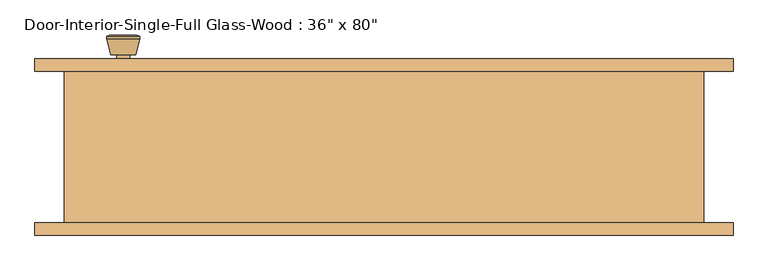
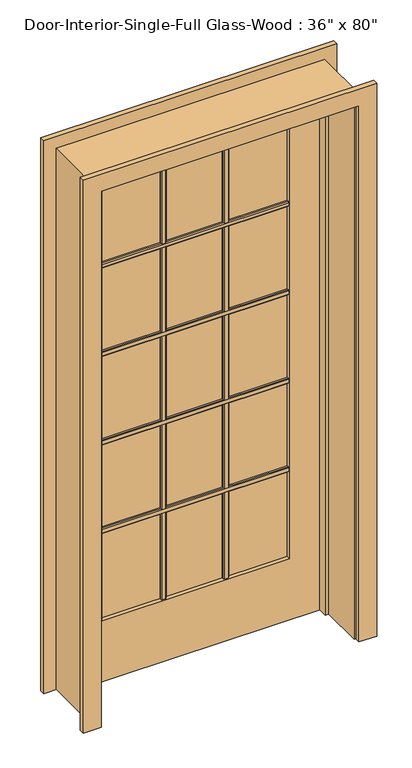
"""IFC4 building model written with IfcOpenShell, lengths in millimetres: door geometry."""

from ifc_helpers import new_model, si_unit, point, frame, frame_2d, origin, place, context, project, spatial, polyline, circle_curve, trimmed, segment, composite_curve, outline, extrude, faceted_brep, source, transform, mapped, element, save
from ifc_brep_helpers import plane_surface, cylinder_surface, revolved_surface, advanced_brep


def door_d5d480c1(model_context):
    return source(origin(), model_context, "Body", "SolidModel", [
        extrude(outline(polyline([(97.155, 1586.23), (103.505, 1586.23), (106.68, 1583.055), (106.68, 1570.355), (103.505, 1567.18), (97.155, 1567.18), (97.155, 1586.23)])), frame((-336.55, 0.0, 0.0), z_axis=(1.0, 0.0, 0.0), x_axis=(0.0, 1.0, 0.0)), (0.0, 0.0, 1.0), 673.1),
        extrude(outline(polyline([(97.155, 1249.9975), (103.505, 1249.9975), (106.68, 1246.8225), (106.68, 1234.1225), (103.505, 1230.9475), (97.155, 1230.9475), (97.155, 1249.9975)])), frame((-336.55, 0.0, 0.0), z_axis=(1.0, 0.0, 0.0), x_axis=(0.0, 1.0, 0.0)), (0.0, 0.0, 1.0), 673.1),
        extrude(outline(polyline([(97.155, 913.765), (103.505, 913.765), (106.68, 910.59), (106.68, 897.89), (103.505, 894.715), (97.155, 894.715), (97.155, 913.765)])), frame((-336.55, 0.0, 0.0), z_axis=(1.0, 0.0, 0.0), x_axis=(0.0, 1.0, 0.0)), (0.0, 0.0, 1.0), 673.1),
        extrude(outline(polyline([(97.155, 577.5325), (103.505, 577.5325), (106.68, 574.3575), (106.68, 561.6575), (103.505, 558.4825), (97.155, 558.4825), (97.155, 577.5325)])), frame((-336.55, 0.0, 0.0), z_axis=(1.0, 0.0, 0.0), x_axis=(0.0, 1.0, 0.0)), (0.0, 0.0, 1.0), 673.1),
        extrude(outline(polyline([(102.6583333, 97.155), (102.6583333, 103.505), (105.8333333, 106.68), (118.5333333, 106.68), (121.7083333, 103.505), (121.7083333, 97.155), (102.6583333, 97.155)])), frame((0.0, 0.0, 231.775), z_axis=(0.0, 0.0, 1.0), x_axis=(1.0, 0.0, 0.0)), (0.0, 0.0, 1.0), 1681.1625),
        extrude(outline(polyline([(-121.7083333, 97.155), (-121.7083333, 103.505), (-118.5333333, 106.68), (-105.8333333, 106.68), (-102.6583333, 103.505), (-102.6583333, 97.155), (-121.7083333, 97.155)])), frame((0.0, 0.0, 231.775), z_axis=(0.0, 0.0, 1.0), x_axis=(1.0, 0.0, 0.0)), (0.0, 0.0, 1.0), 1681.1625),
        extrude(outline(polyline([(90.17, 1586.23), (90.17, 1567.18), (83.82, 1567.18), (80.645, 1570.355), (80.645, 1583.055), (83.82, 1586.23), (90.17, 1586.23)])), frame((-336.55, 0.0, 0.0), z_axis=(1.0, 0.0, 0.0), x_axis=(0.0, 1.0, 0.0)), (0.0, 0.0, 1.0), 673.1),
        extrude(outline(polyline([(90.17, 1249.9975), (90.17, 1230.9475), (83.82, 1230.9475), (80.645, 1234.1225), (80.645, 1246.8225), (83.82, 1249.9975), (90.17, 1249.9975)])), frame((-336.55, 0.0, 0.0), z_axis=(1.0, 0.0, 0.0), x_axis=(0.0, 1.0, 0.0)), (0.0, 0.0, 1.0), 673.1),
        extrude(outline(polyline([(90.17, 913.765), (90.17, 894.715), (83.82, 894.715), (80.645, 897.89), (80.645, 910.59), (83.82, 913.765), (90.17, 913.765)])), frame((-336.55, 0.0, 0.0), z_axis=(1.0, 0.0, 0.0), x_axis=(0.0, 1.0, 0.0)), (0.0, 0.0, 1.0), 673.1),
        extrude(outline(polyline([(90.17, 577.5325), (90.17, 558.4825), (83.82, 558.4825), (80.645, 561.6575), (80.645, 574.3575), (83.82, 577.5325), (90.17, 577.5325)])), frame((-336.55, 0.0, 0.0), z_axis=(1.0, 0.0, 0.0), x_axis=(0.0, 1.0, 0.0)), (0.0, 0.0, 1.0), 673.1),
        extrude(outline(polyline([(102.6583333, 90.17), (121.7083333, 90.17), (121.7083333, 83.82), (118.5333333, 80.645), (105.8333333, 80.645), (102.6583333, 83.82), (102.6583333, 90.17)])), frame((0.0, 0.0, 231.775), z_axis=(0.0, 0.0, 1.0), x_axis=(1.0, 0.0, 0.0)), (0.0, 0.0, 1.0), 1681.1625),
        extrude(outline(polyline([(-121.7083333, 90.17), (-102.6583333, 90.17), (-102.6583333, 83.82), (-105.8333333, 80.645), (-118.5333333, 80.645), (-121.7083333, 83.82), (-121.7083333, 90.17)])), frame((0.0, 0.0, 231.775), z_axis=(0.0, 0.0, 1.0), x_axis=(1.0, 0.0, 0.0)), (0.0, 0.0, 1.0), 1681.1625),
        advanced_brep(
        [(-393.7, 70.2, 914.4), (-383.7, 70.2, 914.4), (-403.7, 70.2, 914.4), (-373.2241324, 21.2, 914.4), (-393.7, 21.2, 914.4), (-414.1758676, 21.2, 914.4), (-368.7, 23.0278681, 914.4), (-418.7, 23.0278681, 914.4), (-368.7, 26.4915463, 914.4), (-418.7, 26.4915463, 914.4), (-375.063764, 51.2, 914.4), (-412.336236, 51.2, 914.4), (-383.7, 51.2, 914.4), (-403.7, 51.2, 914.4)],
        [
            (0, 1),
            (1, 2, circle_curve(frame((-393.7, 70.2, 914.4), z_axis=(0.0, 1.0, 0.0), x_axis=(-1.0, 0.0, 0.0)), 10.0)),
            (2, 0),
            (2, 1, circle_curve(frame((-393.7, 70.2, 914.4), z_axis=(0.0, 1.0, 0.0), x_axis=(-1.0, 0.0, 0.0)), 10.0)),
            (3, 4),
            (4, 5),
            (5, 3, circle_curve(frame((-393.7, 21.2, 914.4), z_axis=(0.0, -1.0, 0.0), x_axis=(-1.0, 0.0, 0.0)), 20.4758676)),
            (3, 5, circle_curve(frame((-393.7, 21.2, 914.4), z_axis=(0.0, -1.0, 0.0), x_axis=(-1.0, 0.0, 0.0)), 20.4758676)),
            (6, 3),
            (5, 7),
            (7, 6, circle_curve(frame((-393.7, 23.0278681, 914.4), z_axis=(0.0, -1.0, 0.0), x_axis=(-1.0, 0.0, 0.0)), 25.0)),
            (6, 7, circle_curve(frame((-393.7, 23.0278681, 914.4), z_axis=(0.0, -1.0, 0.0), x_axis=(-1.0, 0.0, 0.0)), 25.0)),
            (8, 6),
            (7, 9),
            (9, 8, circle_curve(frame((-393.7, 26.4915463, 914.4), z_axis=(0.0, -1.0, 0.0), x_axis=(-1.0, 0.0, 0.0)), 25.0)),
            (8, 9, circle_curve(frame((-393.7, 26.4915463, 914.4), z_axis=(0.0, -1.0, 0.0), x_axis=(-1.0, 0.0, 0.0)), 25.0)),
            (10, 8),
            (9, 11),
            (11, 10, circle_curve(frame((-393.7, 51.2, 914.4), z_axis=(0.0, -1.0, 0.0), x_axis=(-1.0, 0.0, 0.0)), 18.636236)),
            (10, 11, circle_curve(frame((-393.7, 51.2, 914.4), z_axis=(0.0, -1.0, 0.0), x_axis=(-1.0, 0.0, 0.0)), 18.636236)),
            (12, 10),
            (11, 13),
            (13, 12, circle_curve(frame((-393.7, 51.2, 914.4), z_axis=(0.0, -1.0, 0.0), x_axis=(-1.0, 0.0, 0.0)), 10.0)),
            (12, 13, circle_curve(frame((-393.7, 51.2, 914.4), z_axis=(0.0, -1.0, 0.0), x_axis=(-1.0, 0.0, 0.0)), 10.0)),
            (1, 12),
            (13, 2),
        ],
        [
            plane_surface(frame((-393.7, 70.2, 914.4), z_axis=(0.0, 1.0, 0.0), x_axis=(-1.0, 0.0, 0.0))),
            plane_surface(frame((-393.7, 21.2, 914.4), z_axis=(0.0, -1.0, 0.0), x_axis=(-1.0, 0.0, 0.0))),
            revolved_surface(polyline([(-414.1758676, 21.2, 914.4), (-418.7, 23.0278681, 914.4)]), (-393.7, 70.2, 914.4), (0.0, 1.0, 0.0)),
            cylinder_surface(frame((-393.7, 70.2, 914.4), z_axis=(0.0, 1.0, 0.0), x_axis=(-1.0, 0.0, 0.0)), 25.0),
            revolved_surface(polyline([(-418.7, 26.4915463, 914.4), (-412.336236, 51.2, 914.4)]), (-393.7, 70.2, 914.4), (0.0, 1.0, 0.0)),
            plane_surface(frame((-393.7, 51.2, 914.4), z_axis=(0.0, 1.0, 0.0), x_axis=(-1.0, 0.0, 0.0))),
            cylinder_surface(frame((-393.7, 70.2, 914.4), z_axis=(0.0, 1.0, 0.0), x_axis=(-1.0, 0.0, 0.0)), 10.0),
        ],
        [
            (0, [[1, 2, 3]]),
            (0, [[-3, 4, -1]]),
            (1, [[5, 6, 7]]),
            (1, [[-6, -5, 8]]),
            (2, [[9, -7, 10, 11]]),
            (2, [[-10, -8, -9, 12]]),
            (3, [[13, -11, 14, 15]]),
            (3, [[-14, -12, -13, 16]]),
            (4, [[17, -15, 18, 19]]),
            (4, [[-18, -16, -17, 20]]),
            (5, [[21, -19, 22, 23]]),
            (5, [[-22, -20, -21, 24]]),
            (6, [[25, -23, 26, -2]]),
            (6, [[-26, -24, -25, -4]]),
        ],
    ),
        extrude(outline(composite_curve([segment(trimmed(circle_curve(frame_2d((914.4, -393.7)), 30.0), [point((914.4, -423.7))], [point((914.4, -363.7))], False, "CARTESIAN"), True, "CONTINUOUS"), segment(trimmed(circle_curve(frame_2d((914.4, -393.7)), 30.0), [point((914.4, -363.7))], [point((914.4, -423.7))], False, "CARTESIAN"), True, "CONTINUOUS")], self_intersect=False)), frame((0.0, 70.2, 0.0), z_axis=(0.0, 1.0, 0.0), x_axis=(0.0, 0.0, 1.0)), (0.0, 0.0, 1.0), 6.0),
        advanced_brep(
        [(-393.7, 117.125, 914.4), (-403.7, 117.125, 914.4), (-383.7, 117.125, 914.4), (-373.2241324, 166.125, 914.4), (-414.1758676, 166.125, 914.4), (-393.7, 166.125, 914.4), (-368.7, 164.2971319, 914.4), (-418.7, 164.2971319, 914.4), (-368.7, 160.8334537, 914.4), (-418.7, 160.8334537, 914.4), (-375.063764, 136.125, 914.4), (-412.336236, 136.125, 914.4), (-383.7, 136.125, 914.4), (-403.7, 136.125, 914.4)],
        [
            (0, 1),
            (1, 2, circle_curve(frame((-393.7, 117.125, 914.4), z_axis=(0.0, -1.0, 0.0), x_axis=(-1.0, 0.0, 0.0)), 10.0)),
            (2, 0),
            (2, 1, circle_curve(frame((-393.7, 117.125, 914.4), z_axis=(0.0, -1.0, 0.0), x_axis=(-1.0, 0.0, 0.0)), 10.0)),
            (3, 4, circle_curve(frame((-393.7, 166.125, 914.4), z_axis=(0.0, 1.0, 0.0), x_axis=(-1.0, 0.0, 0.0)), 20.4758676)),
            (4, 5),
            (5, 3),
            (4, 3, circle_curve(frame((-393.7, 166.125, 914.4), z_axis=(0.0, 1.0, 0.0), x_axis=(-1.0, 0.0, 0.0)), 20.4758676)),
            (6, 7, circle_curve(frame((-393.7, 164.2971319, 914.4), z_axis=(0.0, 1.0, 0.0), x_axis=(-1.0, 0.0, 0.0)), 25.0)),
            (7, 4),
            (3, 6),
            (7, 6, circle_curve(frame((-393.7, 164.2971319, 914.4), z_axis=(0.0, 1.0, 0.0), x_axis=(-1.0, 0.0, 0.0)), 25.0)),
            (8, 9, circle_curve(frame((-393.7, 160.8334537, 914.4), z_axis=(0.0, 1.0, 0.0), x_axis=(-1.0, 0.0, 0.0)), 25.0)),
            (9, 7),
            (6, 8),
            (9, 8, circle_curve(frame((-393.7, 160.8334537, 914.4), z_axis=(0.0, 1.0, 0.0), x_axis=(-1.0, 0.0, 0.0)), 25.0)),
            (10, 11, circle_curve(frame((-393.7, 136.125, 914.4), z_axis=(0.0, 1.0, 0.0), x_axis=(-1.0, 0.0, 0.0)), 18.636236)),
            (11, 9),
            (8, 10),
            (11, 10, circle_curve(frame((-393.7, 136.125, 914.4), z_axis=(0.0, 1.0, 0.0), x_axis=(-1.0, 0.0, 0.0)), 18.636236)),
            (12, 13, circle_curve(frame((-393.7, 136.125, 914.4), z_axis=(0.0, 1.0, 0.0), x_axis=(-1.0, 0.0, 0.0)), 10.0)),
            (13, 11),
            (10, 12),
            (13, 12, circle_curve(frame((-393.7, 136.125, 914.4), z_axis=(0.0, 1.0, 0.0), x_axis=(-1.0, 0.0, 0.0)), 10.0)),
            (1, 13),
            (12, 2),
        ],
        [
            plane_surface(frame((-393.7, 117.125, 914.4), z_axis=(0.0, -1.0, 0.0), x_axis=(-1.0, 0.0, 0.0))),
            plane_surface(frame((-393.7, 166.125, 914.4), z_axis=(0.0, 1.0, 0.0), x_axis=(-1.0, 0.0, 0.0))),
            revolved_surface(polyline([(-414.1758676, 166.125, 914.4), (-418.7, 164.2971319, 914.4)]), (-393.7, 117.125, 914.4), (0.0, -1.0, 0.0)),
            cylinder_surface(frame((-393.7, 117.125, 914.4), z_axis=(0.0, -1.0, 0.0), x_axis=(-1.0, 0.0, 0.0)), 25.0),
            revolved_surface(polyline([(-418.7, 160.8334537, 914.4), (-412.336236, 136.125, 914.4)]), (-393.7, 117.125, 914.4), (0.0, -1.0, 0.0)),
            plane_surface(frame((-393.7, 136.125, 914.4), z_axis=(0.0, -1.0, 0.0), x_axis=(-1.0, 0.0, 0.0))),
            cylinder_surface(frame((-393.7, 117.125, 914.4), z_axis=(0.0, -1.0, 0.0), x_axis=(-1.0, 0.0, 0.0)), 10.0),
        ],
        [
            (0, [[1, 2, 3]]),
            (0, [[-3, 4, -1]]),
            (1, [[5, 6, 7]]),
            (1, [[8, -7, -6]]),
            (2, [[9, 10, -5, 11]]),
            (2, [[12, -11, -8, -10]]),
            (3, [[13, 14, -9, 15]]),
            (3, [[16, -15, -12, -14]]),
            (4, [[17, 18, -13, 19]]),
            (4, [[20, -19, -16, -18]]),
            (5, [[21, 22, -17, 23]]),
            (5, [[24, -23, -20, -22]]),
            (6, [[-2, 25, -21, 26]]),
            (6, [[-4, -26, -24, -25]]),
        ],
    ),
        extrude(outline(composite_curve([segment(trimmed(circle_curve(frame_2d((914.4, -393.7)), 30.0), [point((914.4, -423.7))], [point((914.4, -363.7))], False, "CARTESIAN"), True, "CONTINUOUS"), segment(trimmed(circle_curve(frame_2d((914.4, -393.7)), 30.0), [point((914.4, -363.7))], [point((914.4, -423.7))], False, "CARTESIAN"), True, "CONTINUOUS")], self_intersect=False)), frame((0.0, 111.125, 0.0), z_axis=(0.0, 1.0, 0.0), x_axis=(0.0, 0.0, 1.0)), (0.0, 0.0, 1.0), 6.0),
        faceted_brep([(482.6, 111.125, 0.0), (482.6, -117.475, 0.0), (457.2, -117.475, 0.0), (457.2, 41.275, 0.0), (444.5, 41.275, 0.0), (444.5, 76.2, 0.0), (457.2, 76.2, 0.0), (457.2, 111.125, 0.0), (482.6, 111.125, 2057.4), (482.6, -117.475, 2057.4), (-482.6, -117.475, 2057.4), (-482.6, -117.475, 0.0), (-457.2, -117.475, 0.0), (-457.2, -117.475, 2032.0), (457.2, -117.475, 2032.0), (457.2, 41.275, 2032.0), (-457.2, 41.275, 2032.0), (-457.2, 41.275, 0.0), (-444.5, 41.275, 0.0), (-444.5, 41.275, 2019.3), (444.5, 41.275, 2019.3), (444.5, 76.2, 2019.3), (-444.5, 76.2, 2019.3), (-444.5, 76.2, 0.0), (-457.2, 76.2, 0.0), (-457.2, 76.2, 2032.0), (457.2, 76.2, 2032.0), (457.2, 111.125, 2032.0), (-457.2, 111.125, 2032.0), (-457.2, 111.125, 0.0), (-482.6, 111.125, 0.0), (-482.6, 111.125, 2057.4)], [[[0, 1, 2, 3, 4, 5, 6, 7]], [[1, 0, 8, 9]], [[2, 1, 9, 10, 11, 12, 13, 14]], [[3, 2, 14, 15]], [[4, 3, 15, 16, 17, 18, 19, 20]], [[5, 4, 20, 21]], [[6, 5, 21, 22, 23, 24, 25, 26]], [[7, 6, 26, 27]], [[0, 7, 27, 28, 29, 30, 31, 8]], [[9, 8, 31, 10]], [[15, 14, 13, 16]], [[21, 20, 19, 22]], [[27, 26, 25, 28]], [[30, 29, 24, 23, 18, 17, 12, 11]], [[10, 31, 30, 11]], [[16, 13, 12, 17]], [[22, 19, 18, 23]], [[28, 25, 24, 29]]]),
        extrude(outline(polyline([(2032.0, -457.2), (0.0, -457.2), (0.0, 457.2), (2032.0, 457.2), (2032.0, -457.2)]), holes=[polyline([(1912.9375, -336.55), (1912.9375, 336.55), (231.775, 336.55), (231.775, -336.55), (1912.9375, -336.55)])]), frame((0.0, 76.2, 0.0), z_axis=(0.0, 1.0, 0.0), x_axis=(0.0, 0.0, 1.0)), (0.0, 0.0, 1.0), 34.925),
        extrude(outline(polyline([(336.55, 90.17), (-336.55, 90.17), (-336.55, 97.155), (336.55, 97.155), (336.55, 90.17)])), frame((0.0, 0.0, 231.775), z_axis=(0.0, 0.0, 1.0), x_axis=(1.0, 0.0, 0.0)), (0.0, 0.0, 1.0), 1681.1625),
        extrude(outline(polyline([(0.0, 463.55), (0.0, 527.05), (2101.85, 527.05), (2101.85, -527.05), (0.0, -527.05), (0.0, -463.55), (2038.35, -463.55), (2038.35, 463.55), (0.0, 463.55)])), frame((0.0, 111.125, 0.0), z_axis=(0.0, 1.0, 0.0), x_axis=(0.0, 0.0, 1.0)), (0.0, 0.0, 1.0), 19.05),
        extrude(outline(polyline([(0.0, 463.55), (0.0, 527.05), (2101.85, 527.05), (2101.85, -527.05), (0.0, -527.05), (0.0, -463.55), (2038.35, -463.55), (2038.35, 463.55), (0.0, 463.55)])), frame((0.0, -136.525, 0.0), z_axis=(0.0, 1.0, 0.0), x_axis=(0.0, 0.0, 1.0)), (0.0, 0.0, 1.0), 19.05),
    ])


if __name__ == "__main__":
    model = new_model("IFC4")
    model_context = context("Model", 3, world=origin())
    ifc_project = project(units=[si_unit("LENGTHUNIT", "METRE", prefix="MILLI")], contexts=[model_context])
    site = spatial("IfcSite", under=ifc_project)
    building = spatial("IfcBuilding", under=site)
    placement = place(None, origin())
    door_shape = door_d5d480c1(model_context)
    element("IfcDoor", 1, ObjectType="Door-Interior-Single-Full Glass-Wood : 36\" x 80\"", at=placement, inside=building, context=model_context, shape_type="MappedRepresentation", body=[
        mapped(door_shape, transform((0.0, 0.0, 0.0), x_axis=(1.0, 0.0, 0.0), y_axis=(0.0, 1.0, 0.0), z_axis=(0.0, 0.0, 1.0))),
    ])
    save(model, "model.ifc")

# Revit data of these elements
# Type "Door-Interior-Single-Full Glass-Wood : 36\" x 80\""
#   Type Mark = "11"
#   Analytic Construction = "Wood frame with single clear glass"
#   Top Rail = 0' - 4 11/16"
#   Thickness = 0' - 1 3/8"
#   Thermal Resistance (R) = 1.0102 (h·ft²·°F)/BTU
#   Swing Angle [instance default] = 90.00°
#   Stiles = 0' - 4 3/4"
#   Rough Width = 3' - 2"
#   Rough Height = 6' - 9"
#   Height = 6' - 8"
#   Width = 3' - 0"
#   Heat Transfer Coefficient (U) = 0.9900 BTU/(h·ft²·°F)
#   Bottom Rail = 0' - 9 1/8"
#   Show Grill [instance default] = yes
#   Trim Material = Cherry
#   Panel Material = Cherry
#   Frame Material = Cherry
#   Door Handle Material = Aluminum
#   Visual Light Transmittance = 0
#   Solar Heat Gain Coefficient = 0
#   Wall Closure = (empty or 0)
#   Function = (empty or 0)
# Element 1 (IfcDoor, "Door-Interior-Single-Full Glass-Wood : 36\" x 80\"")
#   Materials on its faces: "Cherry", "Aluminum", "Glass"
# Materials
#   "Cherry": class "Wood", colour RGB 226 177 128, transparency 0, Description = "Prunus Serotina", Cost = 0
#   "Aluminum": class "Metal", colour RGB 247 247 247, transparency 0, Description = "Aluminum 6061", Cost = 0
#   "Glass": class "Glass", colour RGB 0 128 192, transparency 0.75, Description = "Soda Lime Glass", Cost = 0
